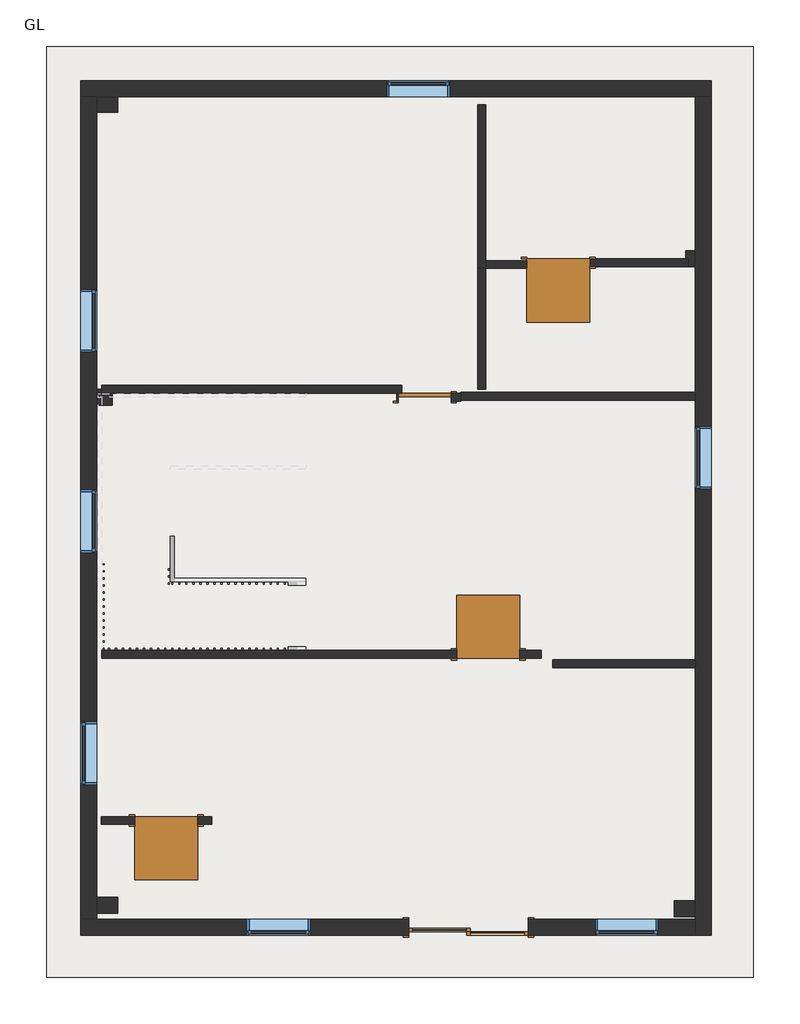
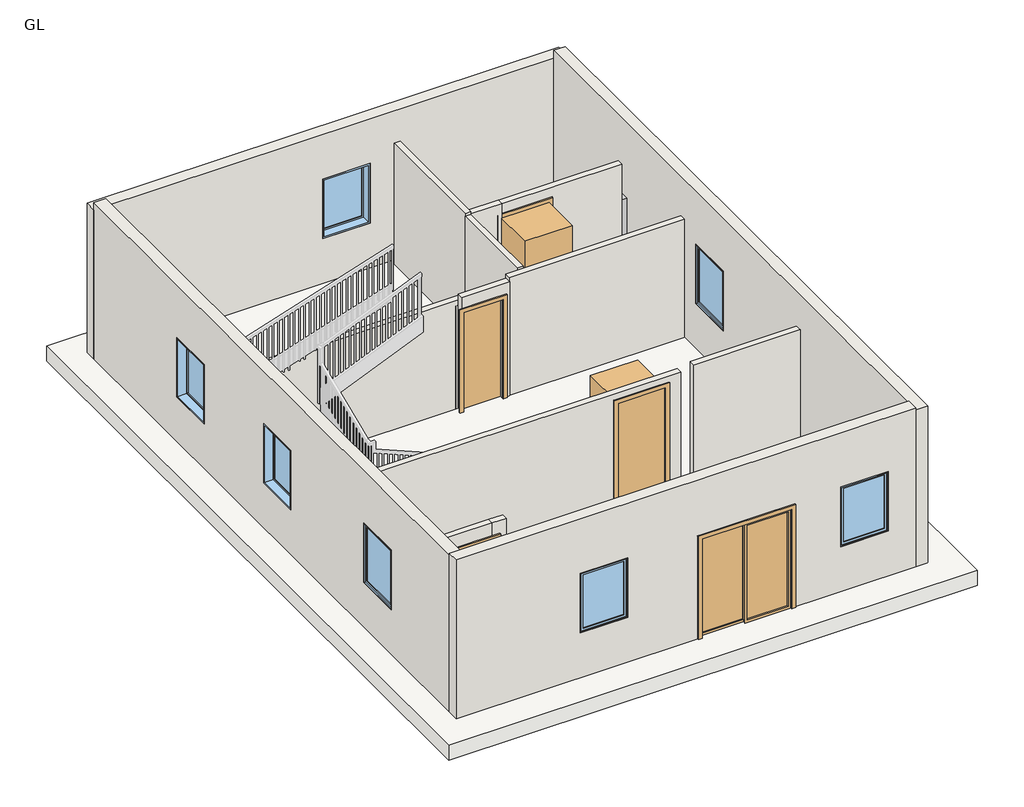
# One storey, part 1 of 3: 15 walls, 7 windows, 5 columns, 5 doors, 1 slab.
"""IFC4 building model written with IfcOpenShell, lengths in millimetres."""

from ifc_helpers import new_model, si_unit, frame, origin, place, context, project, spatial, polyline, outline, extrude, faceted_brep, transform, mapped, element, save
from components import door_ed3b37b7, door_0dbedf7e, door_f2b275c1, fixed_3_x_4_c1f32544

model = new_model("IFC4")

# Units and contexts
model_context = context("Model", 3, world=origin())
ifc_project = project(units=[si_unit("LENGTHUNIT", "METRE", prefix="MILLI")], contexts=[model_context])

# Site, building, storey
site = spatial("IfcSite", under=ifc_project)
building = spatial("IfcBuilding", under=site)
storey = spatial("IfcBuildingStorey", under=building, Name="GL", Elevation=3200.4)

# Columns
placement = place(None, origin())
element("IfcColumn", 1, ObjectType="Rectangular Column : 1'9\"", at=placement, inside=storey, context=model_context, shape_type="SweptSolid", body=[
    extrude(outline(polyline([(10828.4334712, 491.3450307), (10828.4334712, 262.7450307), (10523.6334712, 262.7450307), (10523.6334712, 491.3450307), (10828.4334712, 491.3450307)])), frame((0.0, 0.0, 3200.4), z_axis=(0.0, 0.0, 1.0), x_axis=(1.0, 0.0, 0.0)), (0.0, 0.0, 1.0), 1676.4),
])
element("IfcColumn", 2, ObjectType="Rectangular Column : 1'9\"", at=placement, inside=storey, context=model_context, shape_type="SweptSolid", body=[
    extrude(outline(polyline([(2484.5334712, 542.1450307), (2484.5334712, 313.5450307), (2179.7334712, 313.5450307), (2179.7334712, 542.1450307), (2484.5334712, 542.1450307)])), frame((0.0, 0.0, 3200.4), z_axis=(0.0, 0.0, 1.0), x_axis=(1.0, 0.0, 0.0)), (0.0, 0.0, 1.0), 1676.4),
])
element("IfcColumn", 3, ObjectType="Rectangular Column : 1'9\"", at=placement, inside=storey, context=model_context, shape_type="SweptSolid", body=[
    extrude(outline(polyline([(2408.3334712, 7654.1450307), (2179.7334712, 7654.1450307), (2179.7334712, 7882.7450307), (2255.9334712, 7882.7450307), (2255.9334712, 7825.5950307), (2408.3334712, 7825.5950307), (2408.3334712, 7654.1450307)])), frame((0.0, 0.0, 3200.4), z_axis=(0.0, 0.0, 1.0), x_axis=(1.0, 0.0, 0.0)), (0.0, 0.0, 1.0), 1676.4),
])
element("IfcColumn", 4, ObjectType="Rectangular Column : 1'9\"", at=placement, inside=storey, context=model_context, shape_type="SweptSolid", body=[
    extrude(outline(polyline([(2484.5334712, 12111.8450307), (2484.5334712, 11883.2450307), (2179.7334712, 11883.2450307), (2179.7334712, 12111.8450307), (2484.5334712, 12111.8450307)])), frame((0.0, 0.0, 3200.4), z_axis=(0.0, 0.0, 1.0), x_axis=(1.0, 0.0, 0.0)), (0.0, 0.0, 1.0), 1676.4),
])
element("IfcColumn", 5, ObjectType="Rectangular Column : 1'9\"", at=placement, inside=storey, context=model_context, shape_type="SweptSolid", body=[
    extrude(outline(polyline([(10688.7334712, 9882.9950307), (10828.4334712, 9882.9950307), (10828.4334712, 9654.3950307), (10726.8334712, 9654.3950307), (10726.8334712, 9768.6950307), (10688.7334712, 9768.6950307), (10688.7334712, 9882.9950307)])), frame((0.0, 0.0, 3200.4), z_axis=(0.0, 0.0, 1.0), x_axis=(1.0, 0.0, 0.0)), (0.0, 0.0, 1.0), 1676.4),
])

# Doors
door_shape = door_ed3b37b7(model_context)
element("IfcDoor", 6, ObjectType="Door-Double-Sliding : 68\" x 80\"", at=placement, inside=storey, context=model_context, shape_type="MappedRepresentation", body=[
    mapped(door_shape, transform((7551.8334712, 237.3450307, 3200.4), x_axis=(-1.0, 0.0, 0.0), y_axis=(0.0, -1.0, 0.0), z_axis=(0.0, 0.0, 1.0))),
])
door_2_shape = door_0dbedf7e(model_context)
element("IfcDoor", 7, ObjectType="Single-Flush : 2'8\"X7'", at=placement, inside=storey, context=model_context, shape_type="MappedRepresentation", body=[
    mapped(door_2_shape, transform((7837.5834712, 4053.6950307, 3200.4), x_axis=(1.0, 0.0, 0.0), y_axis=(0.0, 1.0, 0.0), z_axis=(0.0, 0.0, 1.0))),
])
element("IfcDoor", 8, ObjectType="Single-Flush : 2'8\"X7'", at=placement, inside=storey, context=model_context, shape_type="MappedRepresentation", body=[
    mapped(door_2_shape, transform((3184.605209, 1653.3950307, 3200.4), x_axis=(-1.0, 0.0, 0.0), y_axis=(0.0, -1.0, 0.0), z_axis=(0.0, 0.0, 1.0))),
])
element("IfcDoor", 9, ObjectType="Single-Flush : 2'8\"X7'", at=placement, inside=storey, context=model_context, shape_type="MappedRepresentation", body=[
    mapped(door_2_shape, transform((8847.2334712, 9711.5450307, 3200.4), x_axis=(-1.0, 0.0, 0.0), y_axis=(0.0, -1.0, 0.0), z_axis=(0.0, 0.0, 1.0))),
])
door_3_shape = door_f2b275c1(model_context)
element("IfcDoor", 10, ObjectType="Single-Flush : 30\" x 80\"", at=placement, inside=storey, context=model_context, shape_type="MappedRepresentation", body=[
    mapped(door_3_shape, transform((6919.3734712, 7768.4450307, 3200.4), x_axis=(-1.0, 0.0, 0.0), y_axis=(0.0, -1.0, 0.0), z_axis=(0.0, 0.0, 1.0))),
])

# Slab
element("IfcSlab", 11, ObjectType="Generic - 12\"", at=placement, inside=storey, context=model_context, shape_type="SweptSolid", body=[
    extrude(outline(polyline([(11666.6334712, 12835.7450307), (11666.6334712, -613.5549693), (1455.8334712, -613.5549693), (1455.8334712, 12835.7450307), (11666.6334712, 12835.7450307)])), frame((0.0, 0.0, 2895.6), z_axis=(0.0, 0.0, 1.0), x_axis=(1.0, 0.0, 0.0)), (0.0, 0.0, 1.0), 304.8),
])

# Walls
element("IfcWall", 12, ObjectType="Generic - 4.5\"", at=placement, inside=storey, context=model_context, shape_type="Brep", body=[
    faceted_brep([(7437.5334712, 7725.3187832, 3200.4), (10828.4334712, 7725.3187832, 3200.4), (10828.4334712, 7725.3187832, 5612.6250304), (7437.5334712, 7725.3187832, 5612.6250304), (7437.5334712, 7839.6187832, 3200.4), (7437.5334712, 7839.6187832, 5612.6250304), (10828.4334712, 7839.6187832, 5612.6250304), (10828.4334712, 7839.6187832, 3200.4), (7437.5334712, 7825.5950307, 3200.4)], [[[0, 1, 2, 3]], [[4, 5, 6, 7]], [[1, 0, 8, 4, 7]], [[3, 2, 6, 5]], [[0, 3, 5, 4, 8]], [[2, 1, 7, 6]]]),
])
element("IfcWall", 13, ObjectType="Generic - 4.5\"", at=placement, inside=storey, context=model_context, shape_type="Brep", body=[
    faceted_brep([(7685.1834712, 11997.5450307, 3200.4), (7685.1834712, 9628.9950307, 3200.4), (7685.1834712, 9628.9950307, 5617.9045294), (7685.1834712, 9628.9950307, 5672.1996307), (7685.1834712, 11997.5450307, 5672.1996307), (7799.4834712, 11997.5450307, 3200.4), (7799.4834712, 11997.5450307, 5672.1996307), (7799.4834712, 9628.9950307, 5672.1996307), (7799.4834712, 9628.9950307, 5635.757592), (7799.4834712, 9628.9950307, 5617.9045294), (7799.4834712, 9628.9950307, 3200.4), (7799.4834712, 9743.2950307, 3200.4)], [[[0, 1, 2, 3, 4]], [[5, 6, 7, 8, 9, 10, 11]], [[1, 0, 5, 11, 10]], [[4, 3, 7, 6]], [[0, 4, 6, 5]], [[1, 10, 9, 8, 7, 3, 2]]]),
])
element("IfcWall", 14, ObjectType="Generic - 4.5\"", at=placement, inside=storey, context=model_context, shape_type="SweptSolid", body=[
    extrude(outline(polyline([(7799.4834712, 9628.9950307), (7799.4834712, 7882.7450307), (7685.1834712, 7882.7450307), (7685.1834712, 9628.9950307), (7799.4834712, 9628.9950307)])), frame((0.0, 0.0, 3200.4), z_axis=(0.0, 0.0, 1.0), x_axis=(1.0, 0.0, 0.0)), (0.0, 0.0, 1.0), 2417.5045294),
])
element("IfcWall", 15, ObjectType="Generic - 4.5\"", at=placement, inside=storey, context=model_context, shape_type="SweptSolid", body=[
    extrude(outline(polyline([(8390.0334712, 9628.9950307), (7799.4834712, 9628.9950307), (7799.4834712, 9743.2950307), (8390.0334712, 9743.2950307), (8390.0334712, 9628.9950307)])), frame((0.0, 0.0, 3200.4), z_axis=(0.0, 0.0, 1.0), x_axis=(1.0, 0.0, 0.0)), (0.0, 0.0, 1.0), 2435.357592),
])
element("IfcWall", 16, ObjectType="Generic - 4.5\"", at=placement, inside=storey, context=model_context, shape_type="Brep", body=[
    faceted_brep([(10726.8334712, 9654.3950307, 3200.4), (10726.8334712, 9654.3950307, 4876.8), (10726.8334712, 9654.3950307, 5604.5722745), (8390.0334712, 9654.3950307, 5604.5722745), (8390.0334712, 9654.3950307, 5334.0), (9304.4334712, 9654.3950307, 5334.0), (9304.4334712, 9654.3950307, 3200.4), (10726.8334712, 9768.6950307, 5604.5722745), (10726.8334712, 9768.6950307, 4876.8), (10726.8334712, 9768.6950307, 3200.4), (10688.7334712, 9768.6950307, 3200.4), (9304.4334712, 9768.6950307, 3200.4), (9304.4334712, 9768.6950307, 5334.0), (8390.0334712, 9768.6950307, 5334.0), (8390.0334712, 9768.6950307, 5604.5722745)], [[[0, 1, 2, 3, 4, 5, 6]], [[7, 8, 9, 10, 11, 12, 13, 14]], [[9, 0, 6, 11, 10]], [[2, 1, 0, 9, 8, 7]], [[3, 2, 7, 14]], [[3, 14, 13, 4]], [[12, 5, 4, 13]], [[5, 12, 11, 6]]]),
])
element("IfcWall", 17, ObjectType="Generic - 4.5\"", at=placement, inside=storey, context=model_context, shape_type="SweptSolid", body=[
    extrude(outline(polyline([(5667.4443884, 3565.605209), (5667.4443884, 2243.2334712), (3200.4, 2243.2334712), (3200.4, 2727.405209), (5334.0, 2727.405209), (5334.0, 3565.605209), (5667.4443884, 3565.605209)])), frame((0.0, 1596.2450307, 0.0), z_axis=(0.0, 1.0, 0.0), x_axis=(0.0, 0.0, 1.0)), (0.0, 0.0, 1.0), 114.3),
])
element("IfcWall", 18, ObjectType="Generic - 4.5\"", at=placement, inside=storey, context=model_context, shape_type="SweptSolid", body=[
    extrude(outline(polyline([(3200.4, 3843.4334712), (5667.4443884, 3843.4334712), (5667.4443884, 3565.605209), (5334.0, 3565.605209), (5334.0, 3641.805209), (3200.4, 3641.805209), (3200.4, 3843.4334712)])), frame((0.0, 1596.2450307, 0.0), z_axis=(0.0, 1.0, 0.0), x_axis=(0.0, 0.0, 1.0)), (0.0, 0.0, 1.0), 114.3),
])
element("IfcWall", 19, ObjectType="Generic - 4.5\"", at=placement, inside=storey, context=model_context, shape_type="SweptSolid", body=[
    extrude(outline(polyline([(5334.0, 8294.7834712), (3200.4, 8294.7834712), (3200.4, 8599.5834712), (5537.4025818, 8599.5834712), (5537.4025818, 2255.9334712), (3200.4, 2255.9334712), (3200.4, 7380.3834712), (5334.0, 7380.3834712), (5334.0, 8294.7834712)])), frame((0.0, 3996.5450307, 0.0), z_axis=(0.0, 1.0, 0.0), x_axis=(0.0, 0.0, 1.0)), (0.0, 0.0, 1.0), 114.3),
])
element("IfcWall", 20, ObjectType="Generic - 4.5\"", at=placement, inside=storey, context=model_context, shape_type="Brep", body=[
    faceted_brep([(6512.9734712, 7711.2950307, 3200.4), (6538.3734712, 7711.2950307, 3200.4), (6538.3734712, 7711.2950307, 5232.4), (7300.3734712, 7711.2950307, 5232.4), (7300.3734712, 7711.2950307, 3200.4), (7437.5334712, 7711.2950307, 3200.4), (7437.5334712, 7711.2950307, 5534.8745508), (6512.9734712, 7711.2950307, 5534.8745508), (6538.3734712, 7825.5950307, 5232.4), (6538.3734712, 7825.5950307, 3200.4), (6512.9734712, 7825.5950307, 3200.4), (6512.9734712, 7825.5950307, 5534.8745508), (7437.5334712, 7825.5950307, 5534.8745508), (7437.5334712, 7825.5950307, 3200.4), (7300.3734712, 7825.5950307, 3200.4), (7300.3734712, 7825.5950307, 5232.4), (7437.5334712, 7725.3187832, 3200.4)], [[[0, 1, 2, 3, 4, 5, 6, 7]], [[8, 9, 10, 11, 12, 13, 14, 15]], [[14, 13, 16, 5, 4]], [[10, 9, 1, 0]], [[6, 5, 16, 13, 12]], [[7, 6, 12, 11]], [[0, 7, 11, 10]], [[2, 1, 9, 8]], [[3, 2, 8, 15]], [[4, 3, 15, 14]]]),
])
element("IfcWall", 21, ObjectType="Generic - 4.5\"", at=placement, inside=storey, context=model_context, shape_type="SweptSolid", body=[
    extrude(outline(polyline([(10828.4334712, 3860.0200307), (8771.0334712, 3860.0200307), (8771.0334712, 3974.3200307), (10828.4334712, 3974.3200307), (10828.4334712, 3860.0200307)])), frame((0.0, 0.0, 3200.4), z_axis=(0.0, 0.0, 1.0), x_axis=(1.0, 0.0, 0.0)), (0.0, 0.0, 1.0), 2500.2242251),
])
element("IfcWall", 22, ObjectType="Generic - 4.5\"", at=placement, inside=storey, context=model_context, shape_type="Brep", body=[
    faceted_brep([(2255.9334712, 7825.5950307, 3200.4), (2408.3334712, 7825.5950307, 3200.4), (6589.1734712, 7825.5950307, 3200.4), (6589.1734712, 7825.5950307, 5413.9109209), (2255.9334712, 7825.5950307, 5413.9109209), (2255.9334712, 7825.5950307, 4876.8), (2255.9334712, 7939.8950307, 3200.4), (2255.9334712, 7939.8950307, 5413.9109209), (6589.1734712, 7939.8950307, 5413.9109209), (6589.1734712, 7939.8950307, 3200.4), (2255.9334712, 7882.7450307, 3200.4)], [[[0, 1, 2, 3, 4, 5]], [[6, 7, 8, 9]], [[2, 1, 0, 10, 6, 9]], [[3, 2, 9, 8]], [[4, 3, 8, 7]], [[0, 5, 4, 7, 6, 10]]]),
])
element("IfcWall", 23, ObjectType="Generic -9\"", at=placement, inside=storey, context=model_context, shape_type="Brep", body=[
    faceted_brep([(1951.1334712, 12111.8450307, 3200.4), (2179.7334712, 12111.8450307, 3200.4), (2484.5334712, 12111.8450307, 3200.4), (10828.4334712, 12111.8450307, 3200.4), (11057.0334712, 12111.8450307, 3200.4), (11057.0334712, 12111.8450307, 6248.4), (1951.1334712, 12111.8450307, 6248.4), (7285.1334712, 12111.8450307, 5334.0), (7285.1334712, 12111.8450307, 4114.8), (6370.7334712, 12111.8450307, 4114.8), (6370.7334712, 12111.8450307, 5334.0), (1951.1334712, 12340.4450307, 3200.4), (1951.1334712, 12340.4450307, 6248.4), (11057.0334712, 12340.4450307, 6248.4), (11057.0334712, 12340.4450307, 3200.4), (7285.1334712, 12340.4450307, 5334.0), (6370.7334712, 12340.4450307, 5334.0), (6370.7334712, 12340.4450307, 4114.8), (7285.1334712, 12340.4450307, 4114.8)], [[[0, 1, 2, 3, 4, 5, 6], [7, 8, 9, 10]], [[11, 12, 13, 14], [15, 16, 17, 18]], [[4, 3, 2, 1, 0, 11, 14]], [[6, 5, 13, 12]], [[5, 4, 14, 13]], [[0, 6, 12, 11]], [[8, 7, 15, 18]], [[9, 8, 18, 17]], [[10, 9, 17, 16]], [[7, 10, 16, 15]]]),
])
element("IfcWall", 24, ObjectType="Generic -9\"", at=placement, inside=storey, context=model_context, shape_type="Brep", body=[
    faceted_brep([(10828.4334712, 12111.8450307, 3200.4), (10828.4334712, 9882.9950307, 3200.4), (10828.4334712, 9654.3950307, 3200.4), (10828.4334712, 7839.6187832, 3200.4), (10828.4334712, 7725.3187832, 3200.4), (10828.4334712, 3974.3200307, 3200.4), (10828.4334712, 3860.0200307, 3200.4), (10828.4334712, 491.3450307, 3200.4), (10828.4334712, 262.7450307, 3200.4), (10828.4334712, 224.6450307, 3200.4), (10828.4334712, -3.9549693, 3200.4), (10828.4334712, -3.9549693, 6400.8), (10828.4334712, 12111.8450307, 6400.8), (10828.4334712, 7350.6687832, 5334.0), (10828.4334712, 6436.2687832, 5334.0), (10828.4334712, 6436.2687832, 4114.8), (10828.4334712, 7350.6687832, 4114.8), (11057.0334712, 12111.8450307, 3200.4), (11057.0334712, 12111.8450307, 6248.4), (11057.0334712, 12111.8450307, 6400.8), (11057.0334712, -3.9549693, 6400.8), (11057.0334712, -3.9549693, 3200.4), (11057.0334712, 7350.6687832, 5334.0), (11057.0334712, 7350.6687832, 4114.8), (11057.0334712, 6436.2687832, 4114.8), (11057.0334712, 6436.2687832, 5334.0)], [[[0, 1, 2, 3, 4, 5, 6, 7, 8, 9, 10, 11, 12], [13, 14, 15, 16]], [[17, 18, 19, 20, 21], [22, 23, 24, 25]], [[10, 9, 8, 7, 6, 5, 4, 3, 2, 1, 0, 17, 21]], [[12, 11, 20, 19]], [[0, 12, 19, 18, 17]], [[11, 10, 21, 20]], [[23, 22, 13, 16]], [[24, 23, 16, 15]], [[25, 24, 15, 14]], [[22, 25, 14, 13]]]),
])
element("IfcWall", 25, ObjectType="Generic -9\"", at=placement, inside=storey, context=model_context, shape_type="Brep", body=[
    faceted_brep([(6688.2334712, 224.6450307, 5232.4), (6688.2334712, 224.6450307, 3200.4), (2179.7334712, 224.6450307, 3200.4), (1951.1334712, 224.6450307, 3200.4), (1951.1334712, 224.6450307, 6400.8), (1951.1334712, 224.6450307, 6445.3103785), (10828.4334712, 224.6450307, 6445.3103785), (10828.4334712, 224.6450307, 3200.4), (8415.4334712, 224.6450307, 3200.4), (8415.4334712, 224.6450307, 5232.4), (4351.4334712, 224.6450307, 5334.0), (4351.4334712, 224.6450307, 4114.8), (5265.8334712, 224.6450307, 4114.8), (5265.8334712, 224.6450307, 5334.0), (9380.6334712, 224.6450307, 5334.0), (9380.6334712, 224.6450307, 4114.8), (10295.0334712, 224.6450307, 4114.8), (10295.0334712, 224.6450307, 5334.0), (1951.1334712, -3.9549693, 3200.4), (6688.2334712, -3.9549693, 3200.4), (6688.2334712, -3.9549693, 5232.4), (8415.4334712, -3.9549693, 5232.4), (8415.4334712, -3.9549693, 3200.4), (10828.4334712, -3.9549693, 3200.4), (10828.4334712, -3.9549693, 6400.8), (10828.4334712, -3.9549693, 6445.3103785), (1951.1334712, -3.9549693, 6445.3103785), (4351.4334712, -3.9549693, 5334.0), (5265.8334712, -3.9549693, 5334.0), (5265.8334712, -3.9549693, 4114.8), (4351.4334712, -3.9549693, 4114.8), (9380.6334712, -3.9549693, 5334.0), (10295.0334712, -3.9549693, 5334.0), (10295.0334712, -3.9549693, 4114.8), (9380.6334712, -3.9549693, 4114.8)], [[[0, 1, 2, 3, 4, 5, 6, 7, 8, 9], [10, 11, 12, 13], [14, 15, 16, 17]], [[18, 19, 20, 21, 22, 23, 24, 25, 26], [27, 28, 29, 30], [31, 32, 33, 34]], [[8, 7, 23, 22]], [[3, 2, 1, 19, 18]], [[6, 5, 26, 25]], [[7, 6, 25, 24, 23]], [[5, 4, 3, 18, 26]], [[11, 10, 27, 30]], [[12, 11, 30, 29]], [[13, 12, 29, 28]], [[10, 13, 28, 27]], [[15, 14, 31, 34]], [[16, 15, 34, 33]], [[17, 16, 33, 32]], [[14, 17, 32, 31]], [[22, 21, 9, 8]], [[20, 19, 1, 0]], [[21, 20, 0, 9]]]),
])
element("IfcWall", 26, ObjectType="Generic -9\"", at=placement, inside=storey, context=model_context, shape_type="Brep", body=[
    faceted_brep([(2179.7334712, 224.6450307, 3200.4), (2179.7334712, 313.5450307, 3200.4), (2179.7334712, 542.1450307, 3200.4), (2179.7334712, 7654.1450307, 3200.4), (2179.7334712, 7882.7450307, 3200.4), (2179.7334712, 11883.2450307, 3200.4), (2179.7334712, 12111.8450307, 3200.4), (2179.7334712, 12111.8450307, 4876.8), (2179.7334712, 12111.8450307, 6400.8), (2179.7334712, 224.6450307, 6400.8), (2179.7334712, 8416.1450307, 5334.0), (2179.7334712, 9330.5450307, 5334.0), (2179.7334712, 9330.5450307, 4114.8), (2179.7334712, 8416.1450307, 4114.8), (2179.7334712, 5520.5450307, 5334.0), (2179.7334712, 6434.9450307, 5334.0), (2179.7334712, 6434.9450307, 4114.8), (2179.7334712, 5520.5450307, 4114.8), (2179.7334712, 3082.1450307, 5334.0), (2179.7334712, 3082.1450307, 4114.8), (2179.7334712, 2167.7450307, 4114.8), (2179.7334712, 2167.7450307, 5334.0), (1951.1334712, 224.6450307, 3200.4), (1951.1334712, 224.6450307, 6400.8), (1951.1334712, 12111.8450307, 6400.8), (1951.1334712, 12111.8450307, 6248.4), (1951.1334712, 12111.8450307, 3200.4), (1951.1334712, 8416.1450307, 5334.0), (1951.1334712, 8416.1450307, 4114.8), (1951.1334712, 9330.5450307, 4114.8), (1951.1334712, 9330.5450307, 5334.0), (1951.1334712, 5520.5450307, 5334.0), (1951.1334712, 5520.5450307, 4114.8), (1951.1334712, 6434.9450307, 4114.8), (1951.1334712, 6434.9450307, 5334.0), (1951.1334712, 3082.1450307, 5334.0), (1951.1334712, 2167.7450307, 5334.0), (1951.1334712, 2167.7450307, 4114.8), (1951.1334712, 3082.1450307, 4114.8)], [[[0, 1, 2, 3, 4, 5, 6, 7, 8, 9], [10, 11, 12, 13], [14, 15, 16, 17], [18, 19, 20, 21]], [[22, 23, 24, 25, 26], [27, 28, 29, 30], [31, 32, 33, 34], [35, 36, 37, 38]], [[6, 5, 4, 3, 2, 1, 0, 22, 26]], [[9, 8, 24, 23]], [[8, 7, 6, 26, 25, 24]], [[0, 9, 23, 22]], [[28, 27, 10, 13]], [[29, 28, 13, 12]], [[30, 29, 12, 11]], [[27, 30, 11, 10]], [[32, 31, 14, 17]], [[33, 32, 17, 16]], [[34, 33, 16, 15]], [[31, 34, 15, 14]], [[19, 18, 35, 38]], [[20, 19, 38, 37]], [[21, 20, 37, 36]], [[18, 21, 36, 35]]]),
])

# Windows
fixed_3_x_4_shape = fixed_3_x_4_c1f32544(model_context)
element("IfcWindow", 27, ObjectType="Fixed : 3'x 4'", at=placement, inside=storey, context=model_context, shape_type="MappedRepresentation", body=[
    mapped(fixed_3_x_4_shape, transform((4770.5334712, 110.3450307, 3200.4), x_axis=(-1.0, 0.0, 0.0), y_axis=(0.0, -1.0, 0.0), z_axis=(0.0, 0.0, 1.0))),
])
element("IfcWindow", 28, ObjectType="Fixed : 3'x 4'", at=placement, inside=storey, context=model_context, shape_type="MappedRepresentation", body=[
    mapped(fixed_3_x_4_shape, transform((10942.7334712, 6931.5687832, 3200.4), x_axis=(0.0, 1.0, 0.0), y_axis=(-1.0, 0.0, 0.0), z_axis=(0.0, 0.0, 1.0))),
])
element("IfcWindow", 29, ObjectType="Fixed : 3'x 4'", at=placement, inside=storey, context=model_context, shape_type="MappedRepresentation", body=[
    mapped(fixed_3_x_4_shape, transform((6866.0334712, 12226.1450307, 3200.4), x_axis=(1.0, 0.0, 0.0), y_axis=(0.0, 1.0, 0.0), z_axis=(0.0, 0.0, 1.0))),
])
element("IfcWindow", 30, ObjectType="Fixed : 3'x 4'", at=placement, inside=storey, context=model_context, shape_type="MappedRepresentation", body=[
    mapped(fixed_3_x_4_shape, transform((2065.4334712, 8835.2450307, 3200.4), x_axis=(0.0, -1.0, 0.0), y_axis=(1.0, 0.0, 0.0), z_axis=(0.0, 0.0, 1.0))),
])
element("IfcWindow", 31, ObjectType="Fixed : 3'x 4'", at=placement, inside=storey, context=model_context, shape_type="MappedRepresentation", body=[
    mapped(fixed_3_x_4_shape, transform((2065.4334712, 5939.6450307, 3200.4), x_axis=(0.0, -1.0, 0.0), y_axis=(1.0, 0.0, 0.0), z_axis=(0.0, 0.0, 1.0))),
])
element("IfcWindow", 32, ObjectType="Fixed : 3'x 4'", at=placement, inside=storey, context=model_context, shape_type="MappedRepresentation", body=[
    mapped(fixed_3_x_4_shape, transform((2065.4334712, 2663.0450307, 3200.4), x_axis=(0.0, 1.0, 0.0), y_axis=(-1.0, 0.0, 0.0), z_axis=(0.0, 0.0, 1.0))),
])
element("IfcWindow", 33, ObjectType="Fixed : 3'x 4'", at=placement, inside=storey, context=model_context, shape_type="MappedRepresentation", body=[
    mapped(fixed_3_x_4_shape, transform((9799.7334712, 110.3450307, 3200.4), x_axis=(-1.0, 0.0, 0.0), y_axis=(0.0, -1.0, 0.0), z_axis=(0.0, 0.0, 1.0))),
])

save(model, "model.ifc")

# Revit data of these elements
# Type "Rectangular Column : 1'9\""
#   Assembly Code = "B1010200"
#   Depth = 0' - 9"
#   Offset Base = 0' - 0"
#   Offset Top = 0' - 0"
#   Width = 1' - 0"
#   Material = none
# Type "Door-Double-Sliding : 68\" x 80\""
#   Type Mark = "10"
#   Construction Type Id = "opn-d45"
#   Assembly Code = "C1020"
#   Analytic Construction = "Wood frame, double glass door "
#   Thickness = 0' - 2"
#   Thermal Resistance (R) = 1.8150 (h·ft²·°F)/BTU
#   Heat Transfer Coefficient (U) = 0.5510 BTU/(h·ft²·°F)
#   Height = 6' - 8"
#   Rail Width = 0' - 2"
#   Stiles = 0' - 2"
#   Trim Projection Ext = 0' - 1"
#   Trim Projection Int = 0' - 1"
#   Trim Width = 0' - 3"
#   Width = 5' - 8"
#   Define Thermal Properties by = 1
#   Glazing = Glass
#   Panel Material = Wood - Birch - Solid Stained Light Low Gloss
#   Trim Material = Paint - Sienna
#   Visual Light Transmittance = 0
#   Solar Heat Gain Coefficient = 0
#   Function = (empty or 0)
#   Wall Closure = (empty or 0)
# Type "Single-Flush : 2'8\"X7'"
#   Type Mark = "8"
#   Construction Type Id = "MDOOR"
#   Assembly Code = "C1020"
#   Analytic Construction = "Metal"
#   Thickness = 3' - 0"
#   Heat Transfer Coefficient (U) = 0.651978 BTU/(h·ft²·°F)
#   Height = 7' - 0"
#   Trim Projection Ext = 0' - 1"
#   Trim Projection Int = 0' - 1"
#   Trim Width = 0' - 3"
#   Width = 3' - 0"
#   Define Thermal Properties by = 1
#   Door Material = Door - Panel
#   Frame Material = Door - Frame
#   Visual Light Transmittance = 0
#   Solar Heat Gain Coefficient = 0
#   Function = (empty or 0)
#   Wall Closure = (empty or 0)
# Type "Single-Flush : 30\" x 80\""
#   Type Mark = "5"
#   Construction Type Id = "MDOOR"
#   Assembly Code = "C1020"
#   Analytic Construction = "Metal"
#   Thickness = 0' - 2"
#   Heat Transfer Coefficient (U) = 0.651978 BTU/(h·ft²·°F)
#   Height = 6' - 8"
#   Trim Projection Ext = 0' - 1"
#   Trim Projection Int = 0' - 1"
#   Trim Width = 0' - 3"
#   Width = 2' - 6"
#   Define Thermal Properties by = 1
#   Define Thermal Properties by = 1
#   Door Material = Door - Panel
#   Frame Material = Door - Frame
#   Visual Light Transmittance = 0
#   Solar Heat Gain Coefficient = 0
#   Function = (empty or 0)
#   Wall Closure = (empty or 0)
# Type "Generic - 12\""
#   Assembly Code = "B1010"
#   Function = 0
#   Layers, outside or top first: 1' - 0" no material (function 1)
# Type "Generic - 4.5\""
#   Assembly Code = "B2010"
#   Layers, outside or top first: 0' - 4 1/2" no material (function 1)
# Type "Generic -9\""
#   Assembly Code = "B2010"
#   Layers, outside or top first: 0' - 9" no material (function 1)
# Type "Fixed : 3'x 4'"
#   Type Mark = "18"
#   Construction Type Id = "GSP4R"
#   Assembly Code = "B2020100"
#   Analytic Construction = "1/8 in Pilkington single glazing"
#   Visual Light Transmittance = 0.9
#   Solar Heat Gain Coefficient = 0.78
#   Heat Transfer Coefficient (U) = 0.6496 BTU/(h·ft²·°F)
#   Height = 4' - 0"
#   Default Sill Height = 3' - 0"
#   Width = 3' - 0"
#   Window Inset = 0' - 0 3/4"
#   Define Thermal Properties by = 1
#   Glass Pane Material = Glass
#   Sash Material = Sash
#   Wall Closure = (empty or 0)
# Elements 1, 2, 3, 4, 5 (IfcColumn, "Rectangular Column : 1'9\"")
#   Phase Created = New Construction
#   Materials on its faces: "Default Wall"
# Element 6 (IfcDoor, "Door-Double-Sliding : 68\" x 80\"")
#   Phase Created = New Construction
#   Materials on its faces: "Paint - Sienna", "Wood - Birch - Solid Stained Light Low Gloss", "Glass"
# Elements 7, 8, 9 (IfcDoor, "Single-Flush : 2'8\"X7'")
#   Phase Created = New Construction
#   Materials on its faces: "Door - Frame", "Door - Panel"
# Element 10 (IfcDoor, "Single-Flush : 30\" x 80\"")
#   Phase Created = New Construction
#   Materials on its faces: "Door - Frame", "Door - Panel"
# Element 11 (IfcSlab, "Generic - 12\"")
#   Height Offset From Level = 0' - 0"
#   Phase Created = New Construction
#   Materials on its faces: "Default Floor"
# Element 12 (IfcWall, "Generic - 4.5\"")
#   Top Offset = 1' - 10.96949"
#   Base Offset = 0' - 0"
#   Unconnected Height = 7' - 10.96949"
#   wall height = 7' - 10.96949"
#   Phase Created = New Construction
#   Base Constraint = GL
#   Materials on its faces: "Default Wall"
# Element 13 (IfcWall, "Generic - 4.5\"")
#   Top Offset = 2' - 1.31495"
#   Base Offset = 0' - 0"
#   Unconnected Height = 8' - 1.31495"
#   wall height = 8' - 1.31495"
#   Phase Created = New Construction
#   Base Constraint = GL
#   Materials on its faces: "Default Wall"
# Element 14 (IfcWall, "Generic - 4.5\"")
#   Top Offset = 1' - 11.17734"
#   Base Offset = 0' - 0"
#   Unconnected Height = 7' - 11.17734"
#   wall height = 7' - 11.17734"
#   Phase Created = New Construction
#   Base Constraint = GL
#   Materials on its faces: "Default Wall"
# Element 15 (IfcWall, "Generic - 4.5\"")
#   Top Offset = 1' - 11.88022"
#   Base Offset = 0' - 0"
#   Unconnected Height = 7' - 11.88022"
#   wall height = 7' - 11.88022"
#   Phase Created = New Construction
#   Base Constraint = GL
#   Materials on its faces: "Default Wall"
# Element 16 (IfcWall, "Generic - 4.5\"")
#   Top Offset = 1' - 10.65245"
#   Base Offset = 0' - 0"
#   Unconnected Height = 7' - 10.65245"
#   wall height = 7' - 10.65245"
#   Phase Created = New Construction
#   Base Constraint = GL
#   Materials on its faces: "Default Wall"
# Elements 17, 18 (IfcWall, "Generic - 4.5\"")
#   Top Offset = 2' - 1.12773"
#   Base Offset = 0' - 0"
#   Unconnected Height = 8' - 1.12773"
#   wall height = 8' - 1.12773"
#   Phase Created = New Construction
#   Base Constraint = GL
#   Materials on its faces: "Default Wall"
# Element 19 (IfcWall, "Generic - 4.5\"")
#   Top Offset = 1' - 8.00798"
#   Base Offset = 0' - 0"
#   Unconnected Height = 7' - 8.00798"
#   wall height = 7' - 8.00798"
#   Phase Created = New Construction
#   Base Constraint = GL
#   Materials on its faces: "Default Wall"
# Element 20 (IfcWall, "Generic - 4.5\"")
#   Top Offset = 1' - 7.90845"
#   Base Offset = 0' - 0"
#   Unconnected Height = 7' - 7.90845"
#   wall height = 7' - 7.90845"
#   Phase Created = New Construction
#   Base Constraint = GL
#   Materials on its faces: "Default Wall"
# Element 21 (IfcWall, "Generic - 4.5\"")
#   Top Offset = 2' - 2.43402"
#   Base Offset = 0' - 0"
#   Unconnected Height = 8' - 2.43402"
#   wall height = 8' - 2.43402"
#   Phase Created = New Construction
#   Base Constraint = GL
#   Materials on its faces: "Default Wall"
# Element 22 (IfcWall, "Generic - 4.5\"")
#   Top Offset = 1' - 3.1461"
#   Base Offset = 0' - 0"
#   Unconnected Height = 7' - 3.1461"
#   wall height = 7' - 3.1461"
#   Phase Created = New Construction
#   Base Constraint = GL
#   Materials on its faces: "Default Wall"
# Element 23 (IfcWall, "Generic -9\"")
#   Top Offset = 4' - 0"
#   Base Offset = 0' - 0"
#   Unconnected Height = 10' - 0"
#   wall height = 10' - 0"
#   Phase Created = New Construction
#   Base Constraint = GL
#   Materials on its faces: "Default Wall"
# Elements 24, 26 (IfcWall, "Generic -9\"")
#   Top Offset = 0' - 0"
#   Base Offset = 0' - 0"
#   Unconnected Height = 10' - 6"
#   wall height = 10' - 6"
#   Phase Created = New Construction
#   Base Constraint = GL
#   Materials on its faces: "Default Wall"
# Element 25 (IfcWall, "Generic -9\"")
#   Top Offset = 4' - 7.75238"
#   Base Offset = 0' - 0"
#   Unconnected Height = 10' - 7.75238"
#   wall height = 10' - 7.75238"
#   Phase Created = New Construction
#   Base Constraint = GL
#   Materials on its faces: "Default Wall"
# Element 27 (IfcWindow, "Fixed : 3'x 4'")
#   Mark = "8"
#   Phase Created = New Construction
#   Materials on its faces: "Sash", "Glass"
# Element 28 (IfcWindow, "Fixed : 3'x 4'")
#   Mark = "10"
#   Phase Created = New Construction
#   Materials on its faces: "Sash", "Glass"
# Element 29 (IfcWindow, "Fixed : 3'x 4'")
#   Mark = "11"
#   Phase Created = New Construction
#   Materials on its faces: "Sash", "Glass"
# Element 30 (IfcWindow, "Fixed : 3'x 4'")
#   Mark = "12"
#   Phase Created = New Construction
#   Materials on its faces: "Sash", "Glass"
# Element 31 (IfcWindow, "Fixed : 3'x 4'")
#   Mark = "13"
#   Phase Created = New Construction
#   Materials on its faces: "Sash", "Glass"
# Element 32 (IfcWindow, "Fixed : 3'x 4'")
#   Mark = "14"
#   Phase Created = New Construction
#   Materials on its faces: "Sash", "Glass"
# Element 33 (IfcWindow, "Fixed : 3'x 4'")
#   Mark = "15"
#   Phase Created = New Construction
#   Materials on its faces: "Sash", "Glass"
# Materials
#   "Glass": class "Glass", colour RGB 0 128 192, transparency 0.75, Description = "Soda Lime Glass", Cost = 0
#   "Wood - Birch - Solid Stained Light Low Gloss": class "Wood", colour RGB 210 159 95, transparency 0, Cost = 0
#   "Paint - Sienna": colour RGB 118 70 51, transparency 0, Cost = 0
#   "Door - Panel": class "Wood", colour RGB 210 159 95, transparency 0, Cost = 0
#   "Door - Frame": colour RGB 118 70 51, transparency 0, Cost = 0
#   "Sash": class "Wood", colour RGB 224 178 126, transparency 0, Cost = 0
#   "Default Wall": colour RGB 128 128 128, transparency 0, Cost = 0
#   "Default Floor": colour RGB 128 128 128, transparency 0, Cost = 0
